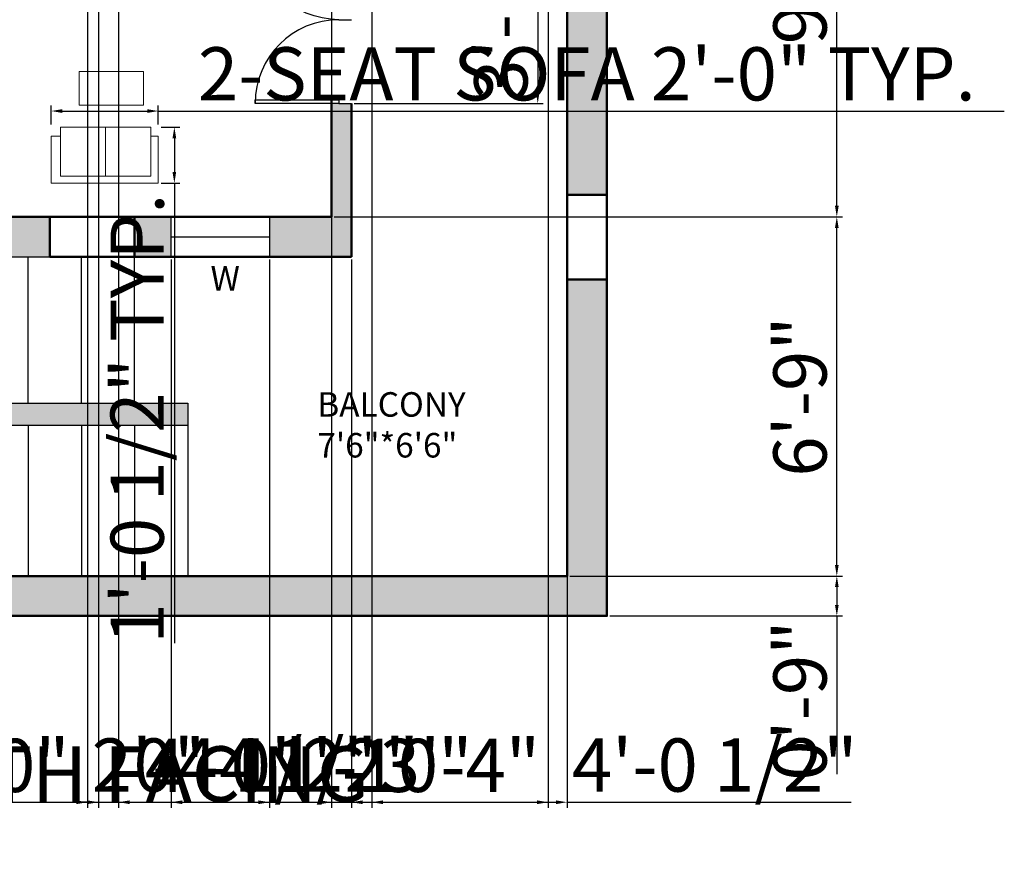
# Model space of a CAD drawing. Units: inches. Extents: x 2063 to 3370, y 2091 to 2971.
# Tile 4 of 14: x 2710 to 2932, y 2091 to 2279. Entities that reach past the tile are written whole.
import ezdxf

# ---------------------------------------------------------------- set-up
doc = ezdxf.new("R2010")
doc.units = ezdxf.units.IN
for name, color, linetype, lineweight in [('A-ANNO-DIMS', 2, 'Continuous', 18), ('A-ANNO-TEXT', 7, 'Continuous', 18), ('A-AREA-IDEN', 3, 'Continuous', 18), ('A-COLS', 7, 'Continuous', 50), ('A-DOOR', 4, 'Continuous', 25), ('A-FLOR-STRS', 3, 'Continuous', 25), ('A-FURN', 8, 'Continuous', 18), ('A-GLAZ', 131, 'Continuous', 25), ('A-WALL', 7, 'Continuous', 50), ('A-WALL-PATT', 8, 'Continuous', 13)]:
    doc.layers.add(name, color=color, linetype=linetype, lineweight=lineweight)
doc.styles.get("Standard").update_dxf_attribs({"font": 'arial.ttf'})
doc.dimstyles.new('ISO-25', dxfattribs={"dimtxt": 12, "dimasz": 2.5, "dimexe": 1.25, "dimexo": 0.625, "dimtad": 1, "dimdec": 0, "dimlunit": 4, "dimtxsty": 'Standard', "dimcen": 2.5, "dimadec": 0, "dimazin": 0, "dimtfac": 1, "dimtdec": 0, "dimtmove": 0, "dimatfit": 3, "dimfxl": 1, "dimarcsym": 0})

# ---------------------------------------------------------------- blocks, each defined once
blk = doc.blocks.new('*U2')
for p, q in [((0, 0), (0, -6)), ((40, 0), (40, -6))]:
    blk.add_line(p, q)
blk.add_lwpolyline([(0, 0), (0, 40), (1.75, 40), (1.75, 0)], close=True)
blk.add_arc((0, 0), 40, 0, 90)
blk = doc.blocks.new('SOFA-2SEAT')
for p, q in [((0, 2.07), (0, 12.63)), ((0, 12.63), (24.16, 12.63)), ((24.16, 12.63), (24.16, 2.07)), ((12.27, 11.03), (12.27, 0)), ((2.08, 2.07), (0, 2.07)), ((24.16, 2.07), (22.46, 2.07))]:
    blk.add_line(p, q)
blk.add_lwpolyline([(22.46, 0), (2.08, 0), (2.08, 11.03), (22.46, 11.03)], close=True)
blk = doc.blocks.new('*D18')
at = {"layer": 'A-ANNO-DIMS', "color": 0, "lineweight": -2, "transparency": 16777216}
for p, q in [((2717.43, 2255.3), (2717.43, 2259.55)), ((2719.93, 2258.3), (2739.08, 2258.3)), ((2741.58, 2255.3), (2741.58, 2259.55)), ((2741.58, 2258.3), (2932.33, 2258.3))]:
    blk.add_line(p, q, dxfattribs=at)
at = {"layer": 'A-ANNO-DIMS', "color": 0, "transparency": 16777216}
for points in [[(2719.93, 2258.72), (2719.93, 2257.88), (2717.43, 2258.3)], [(2739.08, 2258.72), (2739.08, 2257.88), (2741.58, 2258.3)]]:
    blk.add_solid(points, dxfattribs=at)
at = {"layer": 'Defpoints', "color": 0, "transparency": 16777216}
for p in [(2741.58, 2258.3), (2717.43, 2254.68), (2741.58, 2254.68)]:
    blk.add_point(p, dxfattribs=at)
at = {"layer": 'A-ANNO-DIMS', "color": 0, "transparency": 16777216, "insert": (2838.21, 2265.13), "char_height": 12, "attachment_point": 5}
blk.add_mtext('2-SEAT SOFA 2\'-0" TYP.', dxfattribs=at)
blk = doc.blocks.new('*D19')
at = {"layer": 'A-ANNO-DIMS', "color": 0, "lineweight": -2, "transparency": 16777216}
for p, q in [((2742.21, 2254.68), (2746.46, 2254.68)), ((2745.21, 2252.18), (2745.21, 2244.54)), ((2742.21, 2242.04), (2746.46, 2242.04)), ((2745.21, 2242.04), (2745.21, 2138.31))]:
    blk.add_line(p, q, dxfattribs=at)
at = {"layer": 'A-ANNO-DIMS', "color": 0, "transparency": 16777216}
for points in [[(2744.79, 2252.18), (2745.62, 2252.18), (2745.21, 2254.68)], [(2744.79, 2244.54), (2745.62, 2244.54), (2745.21, 2242.04)]]:
    blk.add_solid(points, dxfattribs=at)
at = {"layer": 'Defpoints', "color": 0, "transparency": 16777216}
for p in [(2741.58, 2254.68), (2741.58, 2242.04), (2745.21, 2242.04)]:
    blk.add_point(p, dxfattribs=at)
at = {"layer": 'A-ANNO-DIMS', "color": 0, "transparency": 16777216, "insert": (2738.38, 2188.93), "char_height": 12, "attachment_point": 5, "rotation": 90}
blk.add_mtext('1\'-0 1/2" TYP.', dxfattribs=at)
blk = doc.blocks.new('*D90')
at = {"layer": 'A-ANNO-DIMS', "color": 0, "lineweight": -2, "transparency": 16777216}
for p, q in [((2653.66, 2224.8), (2653.66, 2101.18)), ((2675.81, 2224.8), (2675.81, 2101.18)), ((2656.16, 2102.43), (2673.31, 2102.43)), ((2675.81, 2102.43), (2719.66, 2102.43))]:
    blk.add_line(p, q, dxfattribs=at)
at = {"layer": 'A-ANNO-DIMS', "color": 0, "transparency": 16777216}
for points in [[(2656.16, 2102.84), (2656.16, 2102.01), (2653.66, 2102.43)], [(2673.31, 2102.84), (2673.31, 2102.01), (2675.81, 2102.43)]]:
    blk.add_solid(points, dxfattribs=at)
at = {"layer": 'Defpoints', "color": 0, "transparency": 16777216}
for p in [(2653.66, 2225.43), (2675.81, 2225.43), (2675.81, 2102.43)]:
    blk.add_point(p, dxfattribs=at)
at = {"layer": 'A-ANNO-DIMS', "color": 0, "transparency": 16777216, "insert": (2698.99, 2109.18), "char_height": 12, "attachment_point": 5}
blk.add_mtext('1\'-10"', dxfattribs=at)
blk = doc.blocks.new('*D91')
at = {"layer": 'A-ANNO-DIMS', "color": 0, "lineweight": -2, "transparency": 16777216}
for p, q in [((2744.5, 2224.8), (2744.5, 2101.18)), ((2766.65, 2224.8), (2766.65, 2101.18)), ((2747, 2102.43), (2764.15, 2102.43)), ((2766.65, 2102.43), (2810.5, 2102.43))]:
    blk.add_line(p, q, dxfattribs=at)
at = {"layer": 'A-ANNO-DIMS', "color": 0, "transparency": 16777216}
for points in [[(2747, 2102.84), (2747, 2102.01), (2744.5, 2102.43)], [(2764.15, 2102.84), (2764.15, 2102.01), (2766.65, 2102.43)]]:
    blk.add_solid(points, dxfattribs=at)
at = {"layer": 'Defpoints', "color": 0, "transparency": 16777216}
for p in [(2744.5, 2225.43), (2766.65, 2225.43), (2766.65, 2102.43)]:
    blk.add_point(p, dxfattribs=at)
at = {"layer": 'A-ANNO-DIMS', "color": 0, "transparency": 16777216, "insert": (2789.82, 2109.18), "char_height": 12, "attachment_point": 5}
blk.add_mtext('1\'-10"', dxfattribs=at)
blk = doc.blocks.new('*D93')
at = {"layer": 'A-ANNO-DIMS', "color": 0, "lineweight": -2, "transparency": 16777216}
for p, q in [((2833.75, 2233.8), (2833.75, 2101.18)), ((2785.14, 2224.8), (2785.14, 2101.18)), ((2787.64, 2102.43), (2831.25, 2102.43)), ((2833.75, 2102.43), (2897.84, 2102.43))]:
    blk.add_line(p, q, dxfattribs=at)
at = {"layer": 'A-ANNO-DIMS', "color": 0, "transparency": 16777216}
for points in [[(2787.64, 2102.84), (2787.64, 2102.01), (2785.14, 2102.43)], [(2831.25, 2102.84), (2831.25, 2102.01), (2833.75, 2102.43)]]:
    blk.add_solid(points, dxfattribs=at)
at = {"layer": 'Defpoints', "color": 0, "transparency": 16777216}
for p in [(2833.75, 2234.43), (2785.14, 2225.43), (2833.75, 2102.43)]:
    blk.add_point(p, dxfattribs=at)
at = {"layer": 'A-ANNO-DIMS', "color": 0, "transparency": 16777216, "insert": (2867.04, 2109.26), "char_height": 12, "attachment_point": 5}
blk.add_mtext('4\'-0 1/2"', dxfattribs=at)
blk = doc.blocks.new('*D94')
at = {"layer": 'A-ANNO-DIMS', "color": 0, "lineweight": -2, "transparency": 16777216}
for p, q in [((2611.75, 2347.8), (2611.75, 2101.18)), ((2728.14, 2347.8), (2728.14, 2101.18)), ((2614.25, 2102.43), (2725.64, 2102.43))]:
    blk.add_line(p, q, dxfattribs=at)
at = {"layer": 'A-ANNO-DIMS', "color": 0, "transparency": 16777216}
for points in [[(2614.25, 2102.84), (2614.25, 2102.01), (2611.75, 2102.43)], [(2725.64, 2102.84), (2725.64, 2102.01), (2728.14, 2102.43)]]:
    blk.add_solid(points, dxfattribs=at)
at = {"layer": 'Defpoints', "color": 0, "transparency": 16777216}
for p in [(2611.75, 2348.43), (2728.14, 2348.43), (2728.14, 2102.43)]:
    blk.add_point(p, dxfattribs=at)
at = {"layer": 'A-ANNO-DIMS', "color": 0, "transparency": 16777216, "insert": (2669.94, 2109.26), "char_height": 12, "attachment_point": 5}
blk.add_mtext('9\'-8 1/2"', dxfattribs=at)
blk = doc.blocks.new('*D95')
at = {"layer": 'A-ANNO-DIMS', "color": 0, "lineweight": -2, "transparency": 16777216}
for p, q in [((2728.14, 2347.8), (2728.14, 2101.18)), ((2732.64, 2347.8), (2732.64, 2101.18)), ((2725.64, 2102.43), (2723.14, 2102.43)), ((2728.14, 2102.43), (2732.64, 2102.43)), ((2735.14, 2102.43), (2798.75, 2102.43))]:
    blk.add_line(p, q, dxfattribs=at)
at = {"layer": 'A-ANNO-DIMS', "color": 0, "transparency": 16777216}
for points in [[(2725.64, 2102.84), (2725.64, 2102.01), (2728.14, 2102.43)], [(2735.14, 2102.84), (2735.14, 2102.01), (2732.64, 2102.43)]]:
    blk.add_solid(points, dxfattribs=at)
at = {"layer": 'Defpoints', "color": 0, "transparency": 16777216}
for p in [(2728.14, 2348.43), (2732.64, 2348.43), (2732.64, 2102.43)]:
    blk.add_point(p, dxfattribs=at)
at = {"layer": 'A-ANNO-DIMS', "color": 0, "transparency": 16777216, "insert": (2768.19, 2109.26), "char_height": 12, "attachment_point": 5}
blk.add_mtext('0\'-4 1/2"', dxfattribs=at)
blk = doc.blocks.new('*D96')
at = {"layer": 'A-ANNO-DIMS', "color": 0, "lineweight": -2, "transparency": 16777216}
for p, q in [((2732.64, 2347.8), (2732.64, 2101.18)), ((2780.64, 2347.8), (2780.64, 2101.18)), ((2735.14, 2102.43), (2778.14, 2102.43))]:
    blk.add_line(p, q, dxfattribs=at)
at = {"layer": 'A-ANNO-DIMS', "color": 0, "transparency": 16777216}
for points in [[(2735.14, 2102.84), (2735.14, 2102.01), (2732.64, 2102.43)], [(2778.14, 2102.84), (2778.14, 2102.01), (2780.64, 2102.43)]]:
    blk.add_solid(points, dxfattribs=at)
at = {"layer": 'Defpoints', "color": 0, "transparency": 16777216}
for p in [(2732.64, 2348.43), (2780.64, 2348.43), (2780.64, 2102.43)]:
    blk.add_point(p, dxfattribs=at)
at = {"layer": 'A-ANNO-DIMS', "color": 0, "transparency": 16777216, "insert": (2756.64, 2109.18), "char_height": 12, "attachment_point": 5}
blk.add_mtext('4\'-0"', dxfattribs=at)
blk = doc.blocks.new('*D111')
at = {"layer": 'A-ANNO-DIMS', "color": 0, "lineweight": -2, "transparency": 16777216}
for p, q in [((2834.37, 2153.43), (2895.82, 2153.43)), ((2894.57, 2150.93), (2894.57, 2146.93)), ((2843.37, 2144.43), (2895.82, 2144.43)), ((2894.57, 2144.43), (2894.57, 2108.78))]:
    blk.add_line(p, q, dxfattribs=at)
at = {"layer": 'A-ANNO-DIMS', "color": 0, "transparency": 16777216}
for points in [[(2894.15, 2150.93), (2894.99, 2150.93), (2894.57, 2153.43)], [(2894.15, 2146.93), (2894.99, 2146.93), (2894.57, 2144.43)]]:
    blk.add_solid(points, dxfattribs=at)
at = {"layer": 'Defpoints', "color": 0, "transparency": 16777216}
for p in [(2833.75, 2153.43), (2842.75, 2144.43), (2894.57, 2144.43)]:
    blk.add_point(p, dxfattribs=at)
at = {"layer": 'A-ANNO-DIMS', "color": 0, "transparency": 16777216, "insert": (2887.82, 2125.35), "char_height": 12, "attachment_point": 5, "rotation": 90}
blk.add_mtext('0\'-9"', dxfattribs=at)
blk = doc.blocks.new('*D112')
at = {"layer": 'A-ANNO-DIMS', "color": 0, "lineweight": -2, "transparency": 16777216}
for p, q in [((2781.26, 2234.43), (2895.82, 2234.43)), ((2894.57, 2155.93), (2894.57, 2231.93)), ((2834.37, 2153.43), (2895.82, 2153.43))]:
    blk.add_line(p, q, dxfattribs=at)
at = {"layer": 'A-ANNO-DIMS', "color": 0, "transparency": 16777216}
for points in [[(2894.15, 2231.93), (2894.99, 2231.93), (2894.57, 2234.43)], [(2894.15, 2155.93), (2894.99, 2155.93), (2894.57, 2153.43)]]:
    blk.add_solid(points, dxfattribs=at)
at = {"layer": 'Defpoints', "color": 0, "transparency": 16777216}
for p in [(2780.64, 2234.43), (2894.57, 2234.43), (2833.75, 2153.43)]:
    blk.add_point(p, dxfattribs=at)
at = {"layer": 'A-ANNO-DIMS', "color": 0, "transparency": 16777216, "insert": (2887.82, 2193.93), "char_height": 12, "attachment_point": 5, "rotation": 90}
blk.add_mtext('6\'-9"', dxfattribs=at)
blk = doc.blocks.new('*D113')
at = {"layer": 'A-ANNO-DIMS', "color": 0, "lineweight": -2, "transparency": 16777216}
for p, q in [((2781.26, 2348.43), (2895.82, 2348.43)), ((2894.57, 2236.93), (2894.57, 2345.93)), ((2781.26, 2234.43), (2895.82, 2234.43))]:
    blk.add_line(p, q, dxfattribs=at)
at = {"layer": 'A-ANNO-DIMS', "color": 0, "transparency": 16777216}
for points in [[(2894.15, 2345.93), (2894.99, 2345.93), (2894.57, 2348.43)], [(2894.15, 2236.93), (2894.99, 2236.93), (2894.57, 2234.43)]]:
    blk.add_solid(points, dxfattribs=at)
at = {"layer": 'Defpoints', "color": 0, "transparency": 16777216}
for p in [(2780.64, 2348.43), (2894.57, 2348.43), (2780.64, 2234.43)]:
    blk.add_point(p, dxfattribs=at)
at = {"layer": 'A-ANNO-DIMS', "color": 0, "transparency": 16777216, "insert": (2887.82, 2291.43), "char_height": 12, "attachment_point": 5, "rotation": 90}
blk.add_mtext('9\'-6"', dxfattribs=at)
blk = doc.blocks.new('*D131')
at = {"layer": 'A-ANNO-DIMS', "color": 0, "lineweight": -2, "transparency": 16777216}
for p, q in [((2789.73, 2476.8), (2789.73, 2101.18)), ((2829.49, 2470.78), (2829.49, 2101.18)), ((2792.23, 2102.43), (2826.99, 2102.43))]:
    blk.add_line(p, q, dxfattribs=at)
at = {"layer": 'A-ANNO-DIMS', "color": 0, "transparency": 16777216}
for points in [[(2792.23, 2102.84), (2792.23, 2102.01), (2789.73, 2102.43)], [(2826.99, 2102.84), (2826.99, 2102.01), (2829.49, 2102.43)]]:
    blk.add_solid(points, dxfattribs=at)
at = {"layer": 'Defpoints', "color": 0, "transparency": 16777216}
for p in [(2789.73, 2477.43), (2829.49, 2471.41), (2829.49, 2102.43)]:
    blk.add_point(p, dxfattribs=at)
at = {"layer": 'A-ANNO-DIMS', "color": 0, "transparency": 16777216, "insert": (2809.61, 2109.18), "char_height": 12, "attachment_point": 5}
blk.add_mtext('3\'-4"', dxfattribs=at)
blk = doc.blocks.new('*D132')
at = {"layer": 'A-ANNO-DIMS', "color": 0, "lineweight": -2, "transparency": 16777216}
for p, q in [((2697.29, 2347.55), (2697.29, 2101.18)), ((2725.61, 2347.55), (2725.61, 2101.18)), ((2699.79, 2102.43), (2723.11, 2102.43)), ((2725.61, 2102.43), (2789.42, 2102.43))]:
    blk.add_line(p, q, dxfattribs=at)
at = {"layer": 'A-ANNO-DIMS', "color": 0, "transparency": 16777216}
for points in [[(2699.79, 2102.84), (2699.79, 2102.01), (2697.29, 2102.43)], [(2723.11, 2102.84), (2723.11, 2102.01), (2725.61, 2102.43)]]:
    blk.add_solid(points, dxfattribs=at)
at = {"layer": 'Defpoints', "color": 0, "transparency": 16777216}
for p in [(2697.29, 2348.17), (2725.61, 2348.17), (2725.61, 2102.43)]:
    blk.add_point(p, dxfattribs=at)
at = {"layer": 'A-ANNO-DIMS', "color": 0, "transparency": 16777216, "insert": (2758.77, 2109.26), "char_height": 12, "attachment_point": 5}
blk.add_mtext('2\'-4 1/2"', dxfattribs=at)
blk = doc.blocks.new('*D134')
at = {"layer": 'A-ANNO-DIMS', "color": 0, "lineweight": -2, "transparency": 16777216}
for p, q in [((2785.76, 2297.78), (2828.39, 2297.78)), ((2827.14, 2295.28), (2827.14, 2262.52)), ((2785.76, 2260.02), (2828.39, 2260.02))]:
    blk.add_line(p, q, dxfattribs=at)
at = {"layer": 'A-ANNO-DIMS', "color": 0, "transparency": 16777216}
for points in [[(2826.72, 2295.28), (2827.55, 2295.28), (2827.14, 2297.78)], [(2826.72, 2262.52), (2827.55, 2262.52), (2827.14, 2260.02)]]:
    blk.add_solid(points, dxfattribs=at)
at = {"layer": 'Defpoints', "color": 0, "transparency": 16777216}
for p in [(2785.14, 2297.78), (2785.14, 2260.02), (2827.14, 2260.02)]:
    blk.add_point(p, dxfattribs=at)
at = {"layer": 'A-ANNO-DIMS', "color": 0, "transparency": 16777216, "insert": (2820.38, 2278.9), "char_height": 12, "attachment_point": 5, "rotation": 90}
blk.add_mtext('3\'-2"', dxfattribs=at)

msp = doc.modelspace()

# ---------------------------------------------------------------- hatches: boundary and pattern name
at = {"layer": 'A-WALL-PATT'}
h = msp.add_hatch(color=256, dxfattribs=at)
h.dxf.hatch_style = 1
h.paths.add_polyline_path([(2842.75, 2864.43), (2602.75, 2864.43), (2602.75, 2831.43), (2608.62, 2831.43), (2608.62, 2859.54), (2836.36, 2859.54), (2836.36, 2831.15), (2842.75, 2831.15)])
h.paths.add_polyline_path([(2775.49, 2177.04), (2815.13, 2177.04), (2815.13, 2197.65), (2775.49, 2197.65)], flags=9)
h.paths.add_polyline_path([(2634.18, 2285.75), (2670.81, 2285.75), (2670.81, 2306.35), (2634.18, 2306.35)], flags=9)
h.paths.add_polyline_path([(2701.65, 2293.1), (2755.85, 2293.1), (2755.85, 2313.71), (2701.65, 2313.71)], flags=9)
h.paths.add_polyline_path([(2735.8, 2415.55), (2772.95, 2415.55), (2772.95, 2436.13), (2735.8, 2436.13)], flags=9)
h.paths.add_polyline_path([(2641.75, 2422.21), (2718.67, 2422.21), (2718.67, 2442.82), (2641.75, 2442.82)], flags=9)
h.paths.add_polyline_path([(2710.43, 2552.92), (2764.91, 2552.92), (2764.91, 2573.53), (2710.43, 2573.53)], flags=9)
h.paths.add_polyline_path([(2625.23, 2527.83), (2661.86, 2527.83), (2661.86, 2548.44), (2625.23, 2548.44)], flags=9)
h.paths.add_polyline_path([(2627.53, 2598.16), (2652.13, 2598.16), (2652.13, 2618.77), (2627.53, 2618.77)], flags=9)
h.paths.add_polyline_path([(2646.64, 2696.08), (2723.56, 2696.08), (2723.56, 2716.69), (2646.64, 2716.69)], flags=9)
h.paths.add_polyline_path([(2791.65, 2795.64), (2828.72, 2795.64), (2828.72, 2807.02), (2791.65, 2807.02)], flags=9)
h.paths.add_polyline_path([(2751.88, 2214.78), (2761.93, 2214.78), (2761.93, 2226.17), (2751.88, 2226.17)], flags=9)
h.paths.add_polyline_path([(2664.96, 2215.71), (2675, 2215.71), (2675, 2227.09), (2664.96, 2227.09)], flags=9)
h.paths.add_polyline_path([(2788.26, 2413.43), (2796.17, 2413.43), (2796.17, 2424.82), (2788.26, 2424.82)], flags=9)
h.paths.add_polyline_path([(2728.86, 2795.64), (2765.93, 2795.64), (2765.93, 2807.02), (2728.86, 2807.02)], flags=9)
h.paths.add_polyline_path([(2760.39, 2726.09), (2823.16, 2726.09), (2823.16, 2746.7), (2760.39, 2746.7)], flags=9)
h = msp.add_hatch(color=256, dxfattribs=at)
h.dxf.hatch_style = 1
h.paths.add_polyline_path([(2290.22, 2192.43), (2278.22, 2192.43), (2182.22, 2192.43), (2182.22, 2189.43), (2182.22, 2187.43), (2278.22, 2187.43), (2290.22, 2187.42)])
h.paths.add_polyline_path([(2748.25, 2192.43), (2736.25, 2192.43), (2640.25, 2192.43), (2640.25, 2189.43), (2640.25, 2187.43), (2736.25, 2187.43), (2748.25, 2187.42)], flags=17)
h.paths.add_polyline_path([(2653.66, 2234.43), (2611.75, 2234.43), (2611.75, 2232.93), (2611.75, 2225.43), (2653.66, 2225.43)])
h.paths.add_polyline_path([(2717.13, 2234.43), (2675.81, 2234.43), (2675.81, 2225.43), (2717.13, 2225.43)])
h.paths.add_polyline_path([(2611.75, 2222.57), (2602.75, 2222.57), (2602.75, 2144.43), (2842.75, 2144.43), (2842.75, 2220.3), (2833.75, 2220.3), (2833.75, 2153.43), (2829.39, 2153.43), (2754.78, 2153.43), (2611.75, 2153.43)])
h.paths.add_polyline_path([(2687.64, 2308.91), (2683.14, 2308.91), (2683.14, 2234.43), (2687.64, 2234.43)])
h.paths.add_polyline_path([(2744.5, 2234.43), (2736.25, 2234.43), (2736.25, 2225.43), (2744.5, 2225.43)])
h.paths.add_polyline_path([(2785.14, 2260.02), (2782.31, 2260.02), (2780.64, 2260.02), (2780.64, 2234.43), (2766.65, 2234.43), (2766.65, 2225.43), (2785.14, 2225.43)])
h.paths.add_polyline_path([(2842.75, 2363.93), (2833.75, 2363.93), (2833.75, 2239.41), (2842.75, 2239.41)])
h.paths.add_polyline_path([(2775.49, 2177.04), (2815.13, 2177.04), (2815.13, 2197.65), (2775.49, 2197.65)], flags=25)
h.paths.add_polyline_path([(2634.18, 2285.75), (2670.81, 2285.75), (2670.81, 2306.35), (2634.18, 2306.35)], flags=9)
h.paths.add_polyline_path([(2701.65, 2293.1), (2755.85, 2293.1), (2755.85, 2313.71), (2701.65, 2313.71)], flags=9)
h.paths.add_polyline_path([(2735.8, 2415.55), (2772.95, 2415.55), (2772.95, 2436.13), (2735.8, 2436.13)], flags=9)
h.paths.add_polyline_path([(2641.75, 2422.21), (2718.67, 2422.21), (2718.67, 2442.82), (2641.75, 2442.82)], flags=9)
h.paths.add_polyline_path([(2710.43, 2552.92), (2764.91, 2552.92), (2764.91, 2573.53), (2710.43, 2573.53)], flags=9)
h.paths.add_polyline_path([(2625.23, 2527.83), (2661.86, 2527.83), (2661.86, 2548.44), (2625.23, 2548.44)], flags=9)
h.paths.add_polyline_path([(2627.53, 2598.16), (2652.13, 2598.16), (2652.13, 2618.77), (2627.53, 2618.77)], flags=9)
h.paths.add_polyline_path([(2646.64, 2696.08), (2723.56, 2696.08), (2723.56, 2716.69), (2646.64, 2716.69)], flags=9)
h.paths.add_polyline_path([(2791.65, 2795.64), (2828.72, 2795.64), (2828.72, 2807.02), (2791.65, 2807.02)], flags=9)
h.paths.add_polyline_path([(2751.88, 2214.78), (2761.93, 2214.78), (2761.93, 2226.17), (2751.88, 2226.17)], flags=9)
h.paths.add_polyline_path([(2788.26, 2413.43), (2796.17, 2413.43), (2796.17, 2424.82), (2788.26, 2424.82)], flags=9)
h.paths.add_polyline_path([(2761.97, 2835.24), (2769.88, 2835.24), (2769.88, 2846.62), (2761.97, 2846.62)], flags=9)
h.paths.add_polyline_path([(2675.89, 2833.68), (2685.93, 2833.68), (2685.93, 2845.06), (2675.89, 2845.06)], flags=9)
h.paths.add_polyline_path([(2728.86, 2795.64), (2765.93, 2795.64), (2765.93, 2807.02), (2728.86, 2807.02)], flags=9)
h.paths.add_polyline_path([(2760.39, 2726.09), (2823.16, 2726.09), (2823.16, 2746.7), (2760.39, 2746.7)], flags=9)
h = msp.add_hatch(color=256, dxfattribs=at)
h.dxf.hatch_style = 1
h.paths.add_polyline_path([(2680.75, 2631.93), (2684.44, 2631.93), (2684.44, 2636.43), (2683.1, 2636.43), (2611.75, 2636.43), (2611.75, 2631.93), (2648.72, 2631.93), (2671.75, 2631.93), (2676.25, 2631.93), (2676.25, 2623.58), (2678.23, 2623.58), (2680.75, 2623.58)])
h.paths.add_polyline_path([(2728.75, 2636.43), (2724.44, 2636.43), (2724.44, 2631.93), (2728.75, 2631.93)])
h.paths.add_polyline_path([(2772.02, 2636.43), (2733.25, 2636.43), (2733.25, 2631.93), (2772.02, 2631.93)])
h.paths.add_polyline_path([(2733.25, 2636.43), (2728.75, 2636.43), (2728.75, 2631.93), (2733.25, 2631.93)])
h.paths.add_polyline_path([(2833.75, 2636.43), (2812.02, 2636.43), (2812.02, 2631.93), (2833.75, 2631.93)])
h.paths.add_polyline_path([(2842.75, 2626.16), (2833.75, 2626.16), (2833.75, 2585.28), (2842.75, 2585.28)])
h.paths.add_polyline_path([(2842.75, 2679.03), (2833.75, 2679.03), (2833.75, 2645.28), (2842.75, 2645.28)])
h.paths.add_polyline_path([(2611.75, 2619.52), (2602.75, 2619.52), (2602.75, 2548.5), (2611.75, 2548.5), (2611.75, 2579.43)])
h.paths.add_polyline_path([(2646.64, 2696.08), (2723.56, 2696.08), (2723.56, 2716.69), (2646.64, 2716.69)], flags=9)
h.paths.add_polyline_path([(2791.65, 2795.64), (2828.72, 2795.64), (2828.72, 2807.02), (2791.65, 2807.02)], flags=9)
h.paths.add_polyline_path([(2761.97, 2835.24), (2769.88, 2835.24), (2769.88, 2846.62), (2761.97, 2846.62)], flags=9)
h.paths.add_polyline_path([(2675.89, 2833.68), (2685.93, 2833.68), (2685.93, 2845.06), (2675.89, 2845.06)], flags=9)
h.paths.add_polyline_path([(2728.86, 2795.64), (2765.93, 2795.64), (2765.93, 2807.02), (2728.86, 2807.02)], flags=9)
h.paths.add_polyline_path([(2775.49, 2177.04), (2815.13, 2177.04), (2815.13, 2197.65), (2775.49, 2197.65)], flags=9)
h.paths.add_polyline_path([(2634.18, 2285.75), (2670.81, 2285.75), (2670.81, 2306.35), (2634.18, 2306.35)], flags=9)
h.paths.add_polyline_path([(2701.65, 2293.1), (2755.85, 2293.1), (2755.85, 2313.71), (2701.65, 2313.71)], flags=9)
h.paths.add_polyline_path([(2735.8, 2415.55), (2772.95, 2415.55), (2772.95, 2436.13), (2735.8, 2436.13)], flags=9)
h.paths.add_polyline_path([(2641.75, 2422.21), (2718.67, 2422.21), (2718.67, 2442.82), (2641.75, 2442.82)], flags=9)
h.paths.add_polyline_path([(2710.43, 2552.92), (2764.91, 2552.92), (2764.91, 2573.53), (2710.43, 2573.53)], flags=9)
h.paths.add_polyline_path([(2625.23, 2527.83), (2661.86, 2527.83), (2661.86, 2548.44), (2625.23, 2548.44)], flags=9)
h.paths.add_polyline_path([(2751.88, 2214.78), (2761.93, 2214.78), (2761.93, 2226.17), (2751.88, 2226.17)], flags=9)
h.paths.add_polyline_path([(2664.96, 2215.71), (2675, 2215.71), (2675, 2227.09), (2664.96, 2227.09)], flags=9)
h.paths.add_polyline_path([(2788.26, 2413.43), (2796.17, 2413.43), (2796.17, 2424.82), (2788.26, 2424.82)], flags=9)
h = msp.add_hatch(color=256, dxfattribs=at)
h.dxf.hatch_style = 1
h.paths.add_polyline_path([(2611.75, 2343.93), (2611.75, 2477.43), (2611.75, 2514.15), (2602.75, 2514.15), (2602.75, 2241.68), (2611.75, 2241.68), (2611.75, 2258.43)])
h.paths.add_polyline_path([(2775.49, 2177.04), (2815.13, 2177.04), (2815.13, 2197.65), (2775.49, 2197.65)], flags=9)
h.paths.add_polyline_path([(2735.8, 2415.55), (2772.95, 2415.55), (2772.95, 2436.13), (2735.8, 2436.13)], flags=9)
h.paths.add_polyline_path([(2641.75, 2422.21), (2718.67, 2422.21), (2718.67, 2442.82), (2641.75, 2442.82)], flags=9)
h.paths.add_polyline_path([(2710.43, 2552.92), (2764.91, 2552.92), (2764.91, 2573.53), (2710.43, 2573.53)], flags=9)
h.paths.add_polyline_path([(2625.23, 2527.83), (2661.86, 2527.83), (2661.86, 2548.44), (2625.23, 2548.44)], flags=9)
h.paths.add_polyline_path([(2627.53, 2598.16), (2652.13, 2598.16), (2652.13, 2618.77), (2627.53, 2618.77)], flags=9)
h.paths.add_polyline_path([(2646.64, 2696.08), (2723.56, 2696.08), (2723.56, 2716.69), (2646.64, 2716.69)], flags=9)
h.paths.add_polyline_path([(2791.65, 2795.64), (2828.72, 2795.64), (2828.72, 2807.02), (2791.65, 2807.02)], flags=9)
h.paths.add_polyline_path([(2751.88, 2214.78), (2761.93, 2214.78), (2761.93, 2226.17), (2751.88, 2226.17)], flags=9)
h.paths.add_polyline_path([(2788.26, 2413.43), (2796.17, 2413.43), (2796.17, 2424.82), (2788.26, 2424.82)], flags=9)
h.paths.add_polyline_path([(2761.97, 2835.24), (2769.88, 2835.24), (2769.88, 2846.62), (2761.97, 2846.62)], flags=9)
h.paths.add_polyline_path([(2675.89, 2833.68), (2685.93, 2833.68), (2685.93, 2845.06), (2675.89, 2845.06)], flags=9)
h.paths.add_polyline_path([(2728.86, 2795.64), (2765.93, 2795.64), (2765.93, 2807.02), (2728.86, 2807.02)], flags=9)
h.paths.add_polyline_path([(2760.39, 2726.09), (2823.16, 2726.09), (2823.16, 2746.7), (2760.39, 2746.7)], flags=9)
h = msp.add_hatch(color=256, dxfattribs=at)
h.dxf.hatch_style = 1
h.paths.add_polyline_path([(2785.14, 2468.43), (2780.64, 2468.43), (2780.64, 2429.31), (2785.14, 2429.31)])
h.paths.add_polyline_path([(2842.75, 2525.28), (2833.75, 2525.28), (2833.75, 2523.93), (2833.75, 2466.93), (2833.75, 2383.04), (2842.75, 2383.04)])
h.paths.add_polyline_path([(2789.73, 2477.43), (2680.75, 2477.43), (2680.75, 2579.43), (2680.75, 2589.96), (2678.23, 2589.96), (2676.25, 2589.96), (2676.25, 2583.93), (2667.25, 2583.93), (2611.75, 2583.93), (2611.75, 2579.43), (2671.75, 2579.43), (2676.25, 2579.43), (2676.25, 2477.43), (2611.75, 2477.43), (2611.75, 2468.43), (2728.75, 2468.43), (2789.73, 2468.43), (2789.73, 2471.41)])
h.paths.add_polyline_path([(2710.43, 2552.92), (2764.91, 2552.92), (2764.91, 2573.53), (2710.43, 2573.53)], flags=25)
h.paths.add_polyline_path([(2625.23, 2527.83), (2661.86, 2527.83), (2661.86, 2548.44), (2625.23, 2548.44)], flags=25)
h.paths.add_polyline_path([(2627.53, 2598.16), (2652.13, 2598.16), (2652.13, 2618.77), (2627.53, 2618.77)], flags=9)
h.paths.add_polyline_path([(2646.64, 2696.08), (2723.56, 2696.08), (2723.56, 2716.69), (2646.64, 2716.69)], flags=9)
h.paths.add_polyline_path([(2791.65, 2795.64), (2828.72, 2795.64), (2828.72, 2807.02), (2791.65, 2807.02)], flags=9)
h.paths.add_polyline_path([(2761.97, 2835.24), (2769.88, 2835.24), (2769.88, 2846.62), (2761.97, 2846.62)], flags=9)
h.paths.add_polyline_path([(2675.89, 2833.68), (2685.93, 2833.68), (2685.93, 2845.06), (2675.89, 2845.06)], flags=9)
h.paths.add_polyline_path([(2728.86, 2795.64), (2765.93, 2795.64), (2765.93, 2807.02), (2728.86, 2807.02)], flags=9)
h.paths.add_polyline_path([(2760.39, 2726.09), (2823.16, 2726.09), (2823.16, 2746.7), (2760.39, 2746.7)], flags=9)
h.paths.add_polyline_path([(2775.49, 2177.04), (2815.13, 2177.04), (2815.13, 2197.65), (2775.49, 2197.65)], flags=9)
h.paths.add_polyline_path([(2634.18, 2285.75), (2670.81, 2285.75), (2670.81, 2306.35), (2634.18, 2306.35)], flags=9)
h.paths.add_polyline_path([(2701.65, 2293.1), (2755.85, 2293.1), (2755.85, 2313.71), (2701.65, 2313.71)], flags=9)
h.paths.add_polyline_path([(2641.75, 2422.21), (2718.67, 2422.21), (2718.67, 2442.82), (2641.75, 2442.82)], flags=9)
h.paths.add_polyline_path([(2751.88, 2214.78), (2761.93, 2214.78), (2761.93, 2226.17), (2751.88, 2226.17)], flags=9)
h.paths.add_polyline_path([(2664.96, 2215.71), (2675, 2215.71), (2675, 2227.09), (2664.96, 2227.09)], flags=9)
h.paths.add_polyline_path([(2788.26, 2413.43), (2796.17, 2413.43), (2796.17, 2424.82), (2788.26, 2424.82)], flags=9)
h = msp.add_hatch(color=256, dxfattribs=at)
h.dxf.hatch_style = 1
h.paths.add_polyline_path([(2655.27, 2831.43), (2611.75, 2831.43), (2611.75, 2822.43), (2655.27, 2822.43)])
h.paths.add_polyline_path([(2722.06, 2831.43), (2703.27, 2831.43), (2703.27, 2822.43), (2722.06, 2822.43)])
h.paths.add_polyline_path([(2754.66, 2831.43), (2741.18, 2831.43), (2741.18, 2822.43), (2754.66, 2822.43)])
h.paths.add_polyline_path([(2833.75, 2831.43), (2779.09, 2831.43), (2779.09, 2822.43), (2833.75, 2822.43)])
h.paths.add_polyline_path([(2790.07, 2822.43), (2785.57, 2822.43), (2785.57, 2774.43), (2790.07, 2774.43)])
h.paths.add_polyline_path([(2775.49, 2177.04), (2815.13, 2177.04), (2815.13, 2197.65), (2775.49, 2197.65)], flags=9)
h.paths.add_polyline_path([(2634.18, 2285.75), (2670.81, 2285.75), (2670.81, 2306.35), (2634.18, 2306.35)], flags=9)
h.paths.add_polyline_path([(2701.65, 2293.1), (2755.85, 2293.1), (2755.85, 2313.71), (2701.65, 2313.71)], flags=9)
h.paths.add_polyline_path([(2735.8, 2415.55), (2772.95, 2415.55), (2772.95, 2436.13), (2735.8, 2436.13)], flags=9)
h.paths.add_polyline_path([(2641.75, 2422.21), (2718.67, 2422.21), (2718.67, 2442.82), (2641.75, 2442.82)], flags=9)
h.paths.add_polyline_path([(2710.43, 2552.92), (2764.91, 2552.92), (2764.91, 2573.53), (2710.43, 2573.53)], flags=9)
h.paths.add_polyline_path([(2625.23, 2527.83), (2661.86, 2527.83), (2661.86, 2548.44), (2625.23, 2548.44)], flags=9)
h.paths.add_polyline_path([(2627.53, 2598.16), (2652.13, 2598.16), (2652.13, 2618.77), (2627.53, 2618.77)], flags=9)
h.paths.add_polyline_path([(2646.64, 2696.08), (2723.56, 2696.08), (2723.56, 2716.69), (2646.64, 2716.69)], flags=9)
h.paths.add_polyline_path([(2791.65, 2795.64), (2828.72, 2795.64), (2828.72, 2807.02), (2791.65, 2807.02)], flags=9)
h.paths.add_polyline_path([(2751.88, 2214.78), (2761.93, 2214.78), (2761.93, 2226.17), (2751.88, 2226.17)], flags=9)
h.paths.add_polyline_path([(2664.96, 2215.71), (2675, 2215.71), (2675, 2227.09), (2664.96, 2227.09)], flags=9)
h.paths.add_polyline_path([(2788.26, 2413.43), (2796.17, 2413.43), (2796.17, 2424.82), (2788.26, 2424.82)], flags=9)
h.paths.add_polyline_path([(2728.86, 2795.64), (2765.93, 2795.64), (2765.93, 2807.02), (2728.86, 2807.02)], flags=9)
h.paths.add_polyline_path([(2760.39, 2726.09), (2823.16, 2726.09), (2823.16, 2746.7), (2760.39, 2746.7)], flags=9)

# ---------------------------------------------------------------- linework, layer by layer
at = {"layer": 'A-COLS'}
for points in [[(2833.75, 2239.41), (2842.75, 2239.41), (2842.75, 2220.3), (2833.75, 2220.3)], [(2717.13, 2225.43), (2717.13, 2234.43), (2736.25, 2234.43), (2736.25, 2225.43)]]:
    msp.add_lwpolyline(points, close=True, dxfattribs=at)
at = {"layer": 'A-FLOR-STRS'}
for p, q in [((2611.75, 2225.43), (2736.25, 2225.43)), ((2712.25, 2192.43), (2712.25, 2225.43)), ((2724.25, 2192.43), (2724.25, 2225.43)), ((2736.25, 2192.43), (2736.25, 2225.43)), ((2640.25, 2192.43), (2736.25, 2192.43)), ((2748.25, 2191.04), (2748.25, 2153.43)), ((2640.25, 2187.43), (2736.25, 2187.43)), ((2712.25, 2187.43), (2712.25, 2153.43)), ((2724.25, 2187.43), (2724.25, 2153.43)), ((2736.25, 2187.43), (2736.25, 2153.43))]:
    msp.add_line(p, q, dxfattribs=at)
msp.add_lwpolyline([(2736.25, 2192.43), (2748.25, 2192.43), (2748.25, 2187.42), (2736.25, 2187.42), (2736.25, 2187.43)], dxfattribs=at)
at = {"layer": 'A-FURN'}
msp.add_lwpolyline([(2723.74, 2267.18), (2738.22, 2267.18), (2738.22, 2259.61), (2723.74, 2259.61)], close=True, dxfattribs=at)
at = {"layer": 'A-GLAZ'}
msp.add_line((2744.5, 2229.93), (2766.65, 2229.93), dxfattribs=at)
msp.add_lwpolyline([(2744.5, 2234.43), (2766.65, 2234.43), (2766.65, 2225.43), (2744.5, 2225.43)], close=True, dxfattribs=at)
at = {"layer": 'A-WALL'}
for p, q in [((2780.64, 2278.98), (2780.64, 2278.83)), ((2780.64, 2260.85), (2780.64, 2234.43)), ((2785.14, 2260.02), (2785.14, 2225.43)), ((2717.13, 2234.43), (2611.75, 2234.43)), ((2736.25, 2234.43), (2736.25, 2225.43)), ((2736.25, 2234.43), (2780.64, 2234.43)), ((2736.25, 2225.43), (2785.14, 2225.43)), ((2754.78, 2153.43), (2829.39, 2153.43))]:
    msp.add_line(p, q, dxfattribs=at)
msp.add_lwpolyline([(2602.75, 2144.43), (2842.75, 2144.43), (2842.75, 2864.43), (2602.75, 2864.43)], close=True, dxfattribs=at)
for points in [[(2833.75, 2234.43), (2833.75, 2378.43)], [(2611.75, 2225.43), (2611.75, 2153.43), (2754.78, 2153.43)], [(2829.39, 2153.43), (2833.75, 2153.43), (2833.75, 2225.43)]]:
    msp.add_lwpolyline(points, dxfattribs=at)

# ---------------------------------------------------------------- block references
at = {"layer": 'A-DOOR', "yscale": 0.4719686351156862, "zscale": 0.4719686351156862, "rotation": 90}
for p, xscale in [((2782.31, 2297.78), -0.4719686351156862), ((2782.31, 2260.02), 0.4719686351156862)]:
    msp.add_blockref('*U2', p, dxfattribs=dict(at, xscale=xscale))
at = {"layer": 'A-FURN', "extrusion": (0, 0, -1), "zscale": -1, "rotation": 180}
msp.add_blockref('SOFA-2SEAT', (-2717.43, 2254.68), dxfattribs=at)

# ---------------------------------------------------------------- texts
at = {"layer": 'A-ANNO-TEXT', "attachment_point": 1}
for s, width, gutter_width, heights, insert, char_height in [('W', 106.0361, 27.61, [0], (2753.36, 2223.32), 5.52), ('EAST & NORTH FACING', 239.9528, 62.49, [33.82], (2607.08, 2115.04), 12.498)]:
    msp.add_mtext_dynamic_manual_height_columns(s, width=width, gutter_width=gutter_width, heights=heights, dxfattribs=dict(at, insert=insert, char_height=char_height))
at = {"layer": 'A-AREA-IDEN', "insert": (2777.44, 2194.9), "char_height": 5.523, "attachment_point": 1}
msp.add_mtext_dynamic_manual_height_columns('BALCONY\\P7\'6"*6\'6"', width=106.0361, gutter_width=27.61, heights=[0], dxfattribs=at)

# ---------------------------------------------------------------- dimensions: what is measured, and where the dimension line sits
at = {"layer": 'A-ANNO-DIMS'}
for base, p1, p2, picture, middle in [((2829.49, 2102.43), (2789.73, 2477.43), (2829.49, 2471.41), '*D131', (2809.61, 2109.18)), ((2728.14, 2102.43), (2611.75, 2348.43), (2728.14, 2348.43), '*D94', (2669.94, 2109.26)), ((2725.61, 2102.43), (2697.29, 2348.17), (2725.61, 2348.17), '*D132', (2758.77, 2109.26)), ((2732.64, 2102.43), (2728.14, 2348.43), (2732.64, 2348.43), '*D95', (2768.19, 2109.26)), ((2780.64, 2102.43), (2732.64, 2348.43), (2780.64, 2348.43), '*D96', (2756.64, 2109.18)), ((2833.75, 2102.43), (2785.14, 2225.43), (2833.75, 2234.43), '*D93', (2867.04, 2109.26)), ((2675.8147, 2102.4264), (2653.6648, 2225.4264), (2675.8147, 2225.4264), '*D90', (2698.9861, 2109.1783)), ((2766.6522, 2102.4264), (2744.5024, 2225.4264), (2766.6522, 2225.4264), '*D91', (2789.8236, 2109.1783))]:
    dim = msp.add_linear_dim(base=base, p1=p1, p2=p2, dimstyle='ISO-25', override={"dimdec": 1, "dimlfac": 1, "dimrnd": 0, "dimzin": 1, "dimdsep": 46, "dimlunit": 4, "dimfrac": 2}, dxfattribs=at)
    dim.commit()
    dim.dimension.update_dxf_attribs({"geometry": picture, "text_midpoint": middle})
for base, p1, p2, angle, picture, middle in [((2894.57, 2348.43), (2780.64, 2234.43), (2780.64, 2348.43), 90, '*D113', (2887.82, 2291.43)), ((2827.14, 2260.02), (2785.14, 2297.78), (2785.14, 2260.02), 270, '*D134', (2820.38, 2278.9)), ((2894.57, 2234.43), (2833.75, 2153.43), (2780.64, 2234.43), 90, '*D112', (2887.82, 2193.93)), ((2894.57, 2144.43), (2833.75, 2153.43), (2842.75, 2144.43), 90, '*D111', (2887.82, 2125.35))]:
    dim = msp.add_linear_dim(base=base, p1=p1, p2=p2, angle=angle, dimstyle='ISO-25', override={"dimdec": 1, "dimlfac": 1, "dimrnd": 0, "dimzin": 1, "dimdsep": 46, "dimlunit": 4, "dimfrac": 2}, dxfattribs=at)
    dim.commit()
    dim.dimension.update_dxf_attribs({"geometry": picture, "text_midpoint": middle})
dim = msp.add_linear_dim(base=(2741.5845, 2258.3011), p1=(2717.4277, 2254.6775), p2=(2741.5845, 2254.6775), text='2-SEAT SOFA <> TYP.', dimstyle='ISO-25', override={"dimdec": 1, "dimrnd": 0, "dimzin": 1, "dimlunit": 4, "dimfrac": 2}, dxfattribs=at)
dim.commit()
dim.dimension.update_dxf_attribs({"geometry": '*D18', "text_midpoint": (2838.2088, 2265.1348)})
dim = msp.add_linear_dim(base=(2745.21, 2242.04), p1=(2741.58, 2254.68), p2=(2741.58, 2242.04), angle=270, text='<> TYP.', dimstyle='ISO-25', override={"dimdec": 1, "dimrnd": 0, "dimzin": 1, "dimlunit": 4, "dimfrac": 2}, dxfattribs=at)
dim.commit()
dim.dimension.update_dxf_attribs({"geometry": '*D19', "text_midpoint": (2738.38, 2188.93)})

doc.saveas('drawing.dxf')
